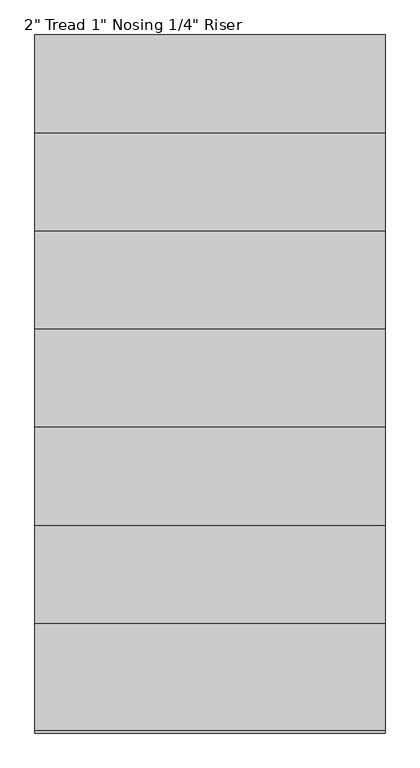
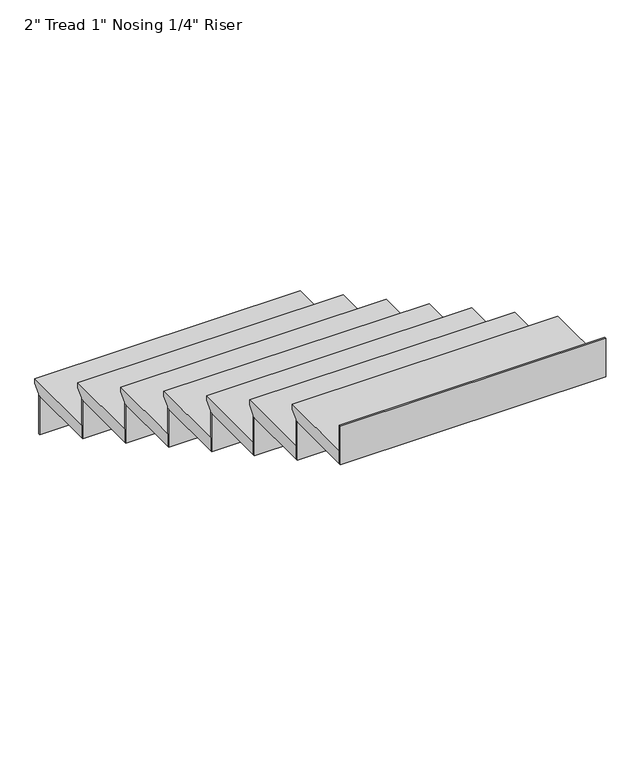
"""IFC4 building model written with IfcOpenShell, lengths in millimetres: stair flight geometry."""

from ifc_helpers import new_model, si_unit, frame, origin, place, context, project, spatial, polyline, outline, extrude, source, transform, mapped, element, save


def stair_flight_2b7c7c02(model_context):
    return source(origin(), model_context, "Body", "SweptSolid", [
        extrude(outline(polyline([(10890.7128362, 5943.6), (11195.5128362, 5943.6), (11195.5128362, 5924.55), (11170.1128362, 5899.15), (11170.1128362, 5892.8), (10890.7128362, 5892.8), (10890.7128362, 5943.6)])), frame((-4958.1002526, 0.0, 0.0), z_axis=(1.0, 0.0, 0.0), x_axis=(0.0, 1.0, 0.0)), (0.0, 0.0, 1.0), 996.95),
        extrude(outline(polyline([(-4958.1002526, 11163.7628362), (-4958.1002526, 11170.1128362), (-3961.1502526, 11170.1128362), (-3961.1502526, 11163.7628362), (-4958.1002526, 11163.7628362)])), frame((0.0, 0.0, 5740.4), z_axis=(0.0, 0.0, 1.0), x_axis=(1.0, 0.0, 0.0)), (0.0, 0.0, 1.0), 152.4),
        extrude(outline(polyline([(-4958.1002526, 10884.3628362), (-4958.1002526, 10890.7128362), (-3961.1502526, 10890.7128362), (-3961.1502526, 10884.3628362), (-4958.1002526, 10884.3628362)])), frame((0.0, 0.0, 5892.8), z_axis=(0.0, 0.0, 1.0), x_axis=(1.0, 0.0, 0.0)), (0.0, 0.0, 1.0), 152.4),
        extrude(outline(polyline([(10611.3128362, 6096.0), (10916.1128362, 6096.0), (10916.1128362, 6076.95), (10890.7128362, 6051.55), (10890.7128362, 6045.2), (10611.3128362, 6045.2), (10611.3128362, 6096.0)])), frame((-4958.1002526, 0.0, 0.0), z_axis=(1.0, 0.0, 0.0), x_axis=(0.0, 1.0, 0.0)), (0.0, 0.0, 1.0), 996.95),
        extrude(outline(polyline([(-4958.1002526, 10604.9628362), (-4958.1002526, 10611.3128362), (-3961.1502526, 10611.3128362), (-3961.1502526, 10604.9628362), (-4958.1002526, 10604.9628362)])), frame((0.0, 0.0, 6045.2), z_axis=(0.0, 0.0, 1.0), x_axis=(1.0, 0.0, 0.0)), (0.0, 0.0, 1.0), 152.4),
        extrude(outline(polyline([(10331.9128362, 6248.4), (10636.7128362, 6248.4), (10636.7128362, 6229.35), (10611.3128362, 6203.95), (10611.3128362, 6197.6), (10331.9128362, 6197.6), (10331.9128362, 6248.4)])), frame((-4958.1002526, 0.0, 0.0), z_axis=(1.0, 0.0, 0.0), x_axis=(0.0, 1.0, 0.0)), (0.0, 0.0, 1.0), 996.95),
        extrude(outline(polyline([(-4958.1002526, 10325.5628362), (-4958.1002526, 10331.9128362), (-3961.1502526, 10331.9128362), (-3961.1502526, 10325.5628362), (-4958.1002526, 10325.5628362)])), frame((0.0, 0.0, 6197.6), z_axis=(0.0, 0.0, 1.0), x_axis=(1.0, 0.0, 0.0)), (0.0, 0.0, 1.0), 152.4),
        extrude(outline(polyline([(10052.5128362, 6400.8), (10357.3128362, 6400.8), (10357.3128362, 6381.75), (10331.9128362, 6356.35), (10331.9128362, 6350.0), (10052.5128362, 6350.0), (10052.5128362, 6400.8)])), frame((-4958.1002526, 0.0, 0.0), z_axis=(1.0, 0.0, 0.0), x_axis=(0.0, 1.0, 0.0)), (0.0, 0.0, 1.0), 996.95),
        extrude(outline(polyline([(-4958.1002526, 10046.1628362), (-4958.1002526, 10052.5128362), (-3961.1502526, 10052.5128362), (-3961.1502526, 10046.1628362), (-4958.1002526, 10046.1628362)])), frame((0.0, 0.0, 6350.0), z_axis=(0.0, 0.0, 1.0), x_axis=(1.0, 0.0, 0.0)), (0.0, 0.0, 1.0), 152.4),
        extrude(outline(polyline([(9773.1128362, 6553.2), (10077.9128362, 6553.2), (10077.9128362, 6534.15), (10052.5128362, 6508.75), (10052.5128362, 6502.4), (9773.1128362, 6502.4), (9773.1128362, 6553.2)])), frame((-4958.1002526, 0.0, 0.0), z_axis=(1.0, 0.0, 0.0), x_axis=(0.0, 1.0, 0.0)), (0.0, 0.0, 1.0), 996.95),
        extrude(outline(polyline([(-4958.1002526, 9766.7628362), (-4958.1002526, 9773.1128362), (-3961.1502526, 9773.1128362), (-3961.1502526, 9766.7628362), (-4958.1002526, 9766.7628362)])), frame((0.0, 0.0, 6502.4), z_axis=(0.0, 0.0, 1.0), x_axis=(1.0, 0.0, 0.0)), (0.0, 0.0, 1.0), 152.4),
        extrude(outline(polyline([(9493.7128362, 6705.6), (9798.5128362, 6705.6), (9798.5128362, 6686.55), (9773.1128362, 6661.15), (9773.1128362, 6654.8), (9493.7128362, 6654.8), (9493.7128362, 6705.6)])), frame((-4958.1002526, 0.0, 0.0), z_axis=(1.0, 0.0, 0.0), x_axis=(0.0, 1.0, 0.0)), (0.0, 0.0, 1.0), 996.95),
        extrude(outline(polyline([(-4958.1002526, 9487.3628362), (-4958.1002526, 9493.7128362), (-3961.1502526, 9493.7128362), (-3961.1502526, 9487.3628362), (-4958.1002526, 9487.3628362)])), frame((0.0, 0.0, 6654.8), z_axis=(0.0, 0.0, 1.0), x_axis=(1.0, 0.0, 0.0)), (0.0, 0.0, 1.0), 152.4),
        extrude(outline(polyline([(-4958.1002526, 9207.9628362), (-4958.1002526, 9214.3128362), (-3961.1502526, 9214.3128362), (-3961.1502526, 9207.9628362), (-4958.1002526, 9207.9628362)])), frame((0.0, 0.0, 6807.2), z_axis=(0.0, 0.0, 1.0), x_axis=(1.0, 0.0, 0.0)), (0.0, 0.0, 1.0), 152.4),
        extrude(outline(polyline([(9214.3128362, 6858.0), (9519.1128362, 6858.0), (9519.1128362, 6838.95), (9493.7128362, 6813.55), (9493.7128362, 6807.2), (9214.3128362, 6807.2), (9214.3128362, 6858.0)])), frame((-4958.1002526, 0.0, 0.0), z_axis=(1.0, 0.0, 0.0), x_axis=(0.0, 1.0, 0.0)), (0.0, 0.0, 1.0), 996.95),
    ])


if __name__ == "__main__":
    model = new_model("IFC4")
    model_context = context("Model", 3, world=origin())
    ifc_project = project(units=[si_unit("LENGTHUNIT", "METRE", prefix="MILLI")], contexts=[model_context])
    site = spatial("IfcSite", under=ifc_project)
    building = spatial("IfcBuilding", under=site)
    placement = place(None, origin())
    stair_flight_shape = stair_flight_2b7c7c02(model_context)
    element("IfcStairFlight", 1, ObjectType="2\" Tread 1\" Nosing 1/4\" Riser", at=placement, inside=building, context=model_context, shape_type="MappedRepresentation", body=[
        mapped(stair_flight_shape, transform((0.0, 0.0, 0.0), x_axis=(1.0, 0.0, 0.0), y_axis=(0.0, 1.0, 0.0), z_axis=(0.0, 0.0, 1.0))),
    ])
    save(model, "model.ifc")
